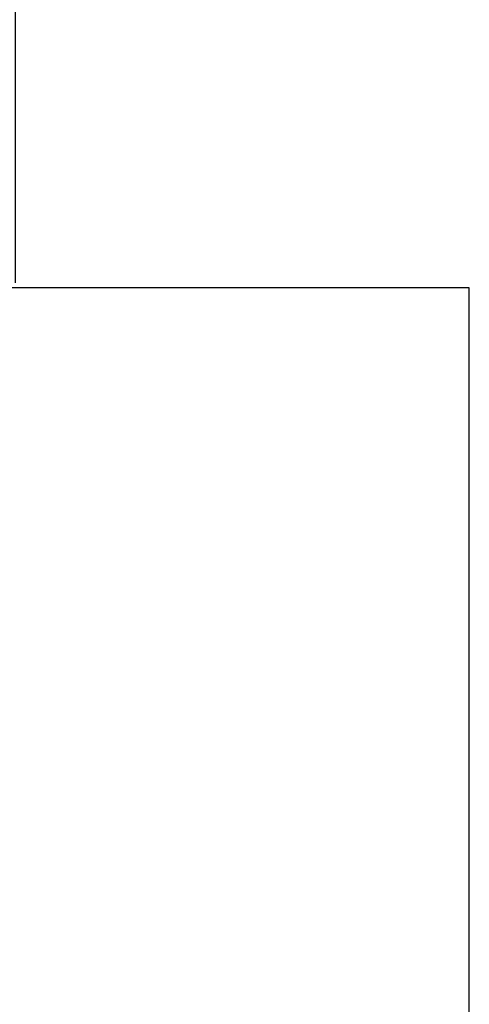
# Model space of a CAD drawing. Units: inches. Extents: x -1198 to -69, y -512 to 437.
# Tile 14 of 50: x -945.11 to -939.4, y 176.14 to 188.63. Entities that reach past the tile are written whole.
import ezdxf

# ---------------------------------------------------------------- set-up
doc = ezdxf.new("R2010")
doc.units = ezdxf.units.IN
doc.header["$MEASUREMENT"] = 0
doc.layers.add('A-ANNO-DIMS', color=2, linetype='Continuous', lineweight=18)
doc.layers.add('A-FLOR-CASE', color=7, linetype='Continuous', lineweight=25)
doc.styles.get("Standard").update_dxf_attribs({"font": 'arial.ttf'})
doc.dimstyles.get("Standard").update_dxf_attribs({"dimtxt": 6, "dimasz": 6, "dimexe": 0.18, "dimexo": 0.0625, "dimgap": 0.09, "dimtad": 0, "dimtih": 1, "dimtoh": 1, "dimdec": 0, "dimzin": 0, "dimdsep": 46, "dimlunit": 4, "dimtxsty": 'Standard', "dimblk": 'OBLIQUE', "dimcen": 0.09, "dimadec": 0, "dimazin": 0, "dimtfac": 1, "dimtdec": 0, "dimtofl": 0, "dimtmove": 0, "dimatfit": 3, "dimfxl": 1, "dimtolj": 1, "dimtzin": 0, "dimarcsym": 0})

# ---------------------------------------------------------------- blocks, each defined once
blk = doc.blocks.new('COUNTER-L')
at = {"ltscale": 10}
for p, q in [((49.349, 24), (0, 24)), ((49.349, 0), (49.349, 24))]:
    blk.add_line(p, q, dxfattribs=at)
blk = doc.blocks.new('_Oblique')
at = {"color": 0, "linetype": 'ByBlock', "lineweight": -2}
blk.add_line((-0.5, -0.5), (0.5, 0.5), dxfattribs=at)
blk = doc.blocks.new('*D50')
at = {"layer": 'A-ANNO-DIMS', "color": 0, "lineweight": -2, "ltscale": 10, "transparency": 16777216}
for p, q in [((-978.462, 185.29), (-978.462, 190.403)), ((-945.163, 185.29), (-945.163, 190.403)), ((-978.462, 190.223), (-984.462, 190.223)), ((-945.163, 190.223), (-978.462, 190.223))]:
    blk.add_line(p, q, dxfattribs=at)
at = {"layer": 'DEFPOINTS', "color": 0, "ltscale": 10, "transparency": 16777216}
for p in [(-978.462, 190.223), (-978.462, 185.228), (-945.163, 185.228)]:
    blk.add_point(p, dxfattribs=at)
at = {"layer": 'A-ANNO-DIMS', "color": 0, "lineweight": -2, "ltscale": 10, "transparency": 16777216, "xscale": 6, "yscale": 6, "zscale": 6, "rotation": 180}
blk.add_blockref('_Oblique', (-978.462, 190.223), dxfattribs=at)
at = {"layer": 'A-ANNO-DIMS', "color": 0, "lineweight": -2, "ltscale": 10, "transparency": 16777216, "xscale": 6, "yscale": 6, "zscale": 6}
blk.add_blockref('_Oblique', (-945.163, 190.223), dxfattribs=at)
at = {"layer": 'A-ANNO-DIMS', "color": 0, "ltscale": 10, "transparency": 16777216, "insert": (-1009.24, 190.223), "char_height": 6, "attachment_point": 5}
blk.add_mtext('\\A1;HOB 33 TYP.', dxfattribs=at)

msp = doc.modelspace()

# ---------------------------------------------------------------- block references
at = {"layer": 'A-FLOR-CASE'}
msp.add_blockref('COUNTER-L', (-988.751, 161.228), dxfattribs=at)

# ---------------------------------------------------------------- dimensions: what is measured, and where the dimension line sits
at = {"layer": 'A-ANNO-DIMS', "ltscale": 10}
dim = msp.add_linear_dim(base=(-978.4621, 190.2226), p1=(-945.1627, 185.2277), p2=(-978.4621, 185.2277), angle=180, text='HOB <> TYP.', dimstyle='Standard', override={"dimdec": 0, "dimlfac": 1, "dimrnd": 0, "dimzin": 0, "dimdsep": 46, "dimlunit": 2}, dxfattribs=at)
dim.commit()
dim.dimension.update_dxf_attribs({"geometry": '*D50', "text_midpoint": (-1009.2397, 190.2226)})

doc.saveas('drawing.dxf')
